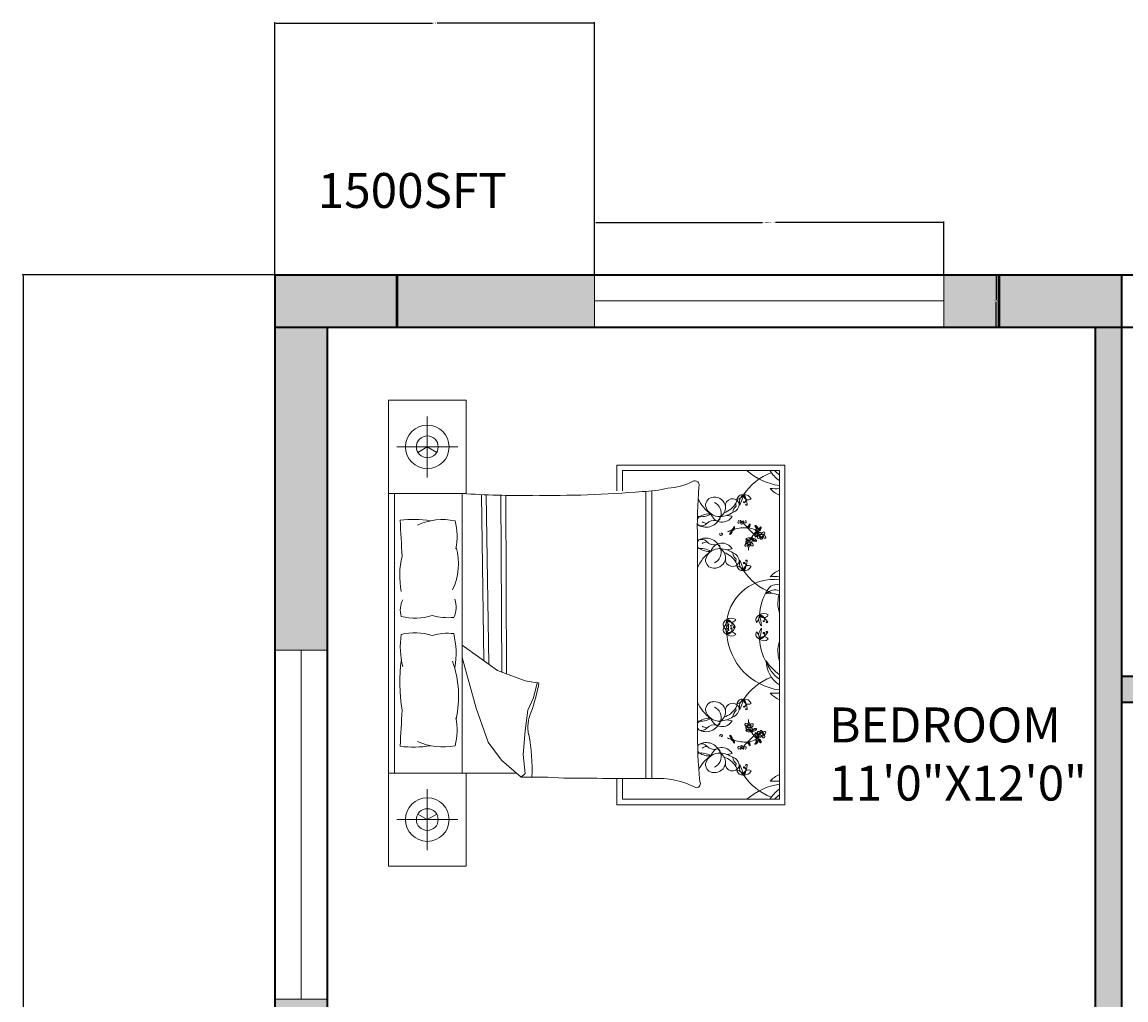
# Model space of a CAD drawing. Units: inches. Extents: x -28 to 485, y -861 to 54.
# Tile 10 of 14: x -28 to 162, y -115 to 54. Entities that reach past the tile are written whole.
import ezdxf

# ---------------------------------------------------------------- set-up
doc = ezdxf.new("R2010")
doc.units = ezdxf.units.IN
doc.header["$MEASUREMENT"] = 0
for name, color, linetype, lineweight in [('A-ANNO-DIMS', 2, 'Continuous', 18), ('A-AREA-IDEN', 7, 'Continuous', 18), ('A-COLS', 7, 'Continuous', 50), ('A-COLS-PATT', 8, 'Continuous', 13), ('A-FURN', 8, 'Continuous', 13), ('A-GLAZ', 4, 'Continuous', 18), ('A-WALL', 7, 'Continuous', 35), ('A-WALL-PATT', 34, 'Continuous', 13)]:
    doc.layers.add(name, color=color, linetype=linetype, lineweight=lineweight)
doc.styles.get("Standard").update_dxf_attribs({"font": 'arial.ttf'})
doc.dimstyles.get("Standard").update_dxf_attribs({"dimtxt": 0.18, "dimasz": 0.18, "dimexe": 0.18, "dimexo": 0.0625, "dimgap": 0.09, "dimtad": 0, "dimtih": 1, "dimtoh": 1, "dimdec": 0, "dimzin": 0, "dimdsep": 46, "dimlunit": 3, "dimtxsty": 'Standard', "dimcen": 0.09, "dimadec": 0, "dimazin": 0, "dimtfac": 1, "dimtdec": 0, "dimtofl": 0, "dimtmove": 0, "dimatfit": 3, "dimfxl": 1, "dimtolj": 1, "dimtzin": 0, "dimarcsym": 0})

# ---------------------------------------------------------------- blocks, each defined once
blk = doc.blocks.new('BED-DOUBLE-WITH-NIGHTSTANDS')
for p, q in [((0, 0), (0, 80.08)), ((6.67, 66.84), (6.67, 77.31)), ((11.91, 72.08), (1.44, 72.08)), ((39.26, 64.51), (39.26, 68.96)), ((39.26, 68.96), (68.11, 68.96)), ((68.11, 68.96), (68.11, 10.57)), ((40.19, 68.03), (40.19, 64.5)), ((67.18, 68.03), (40.19, 68.03)), ((67.18, 11.5), (67.18, 68.03)), ((45.25, 64.51), (45.25, 15.09)), ((1.03, 64.07), (1.03, 16.02)), ((12.66, 16.02), (12.66, 64.07)), ((15.98, 63.85), (16.38, 35.34)), ((16.8, 63.82), (17.22, 34.74)), ((19.33, 63.78), (19.45, 33.37)), ((20.15, 63.78), (20.27, 33.06)), ((44.25, 64.43), (44.25, 15.09)), ((59.06, 60.14), (58.15, 60.31)), ((53.12, 56.3), (53.12, 23.78)), ((59.06, 54.54), (58.15, 54.36)), ((12.66, 38.02), (18.76, 33.63)), ((15.04, 27.14), (12.66, 35.87)), ((18.76, 33.63), (23.47, 31.84)), ((23.47, 31.84), (25.57, 31.52)), ((25.57, 31.52), (24.92, 28.93)), ((24.92, 28.93), (23.95, 26.82)), ((17.14, 21.3), (15.04, 27.14)), ((23.95, 26.82), (23.47, 23.25)), ((59.06, 24.99), (58.15, 25.16)), ((23.47, 23.25), (23.14, 19.19)), ((19.41, 18.22), (17.14, 21.3)), ((23.14, 19.19), (23.47, 15.95)), ((59.06, 19.39), (58.15, 19.21)), ((22.82, 15.3), (19.41, 18.22)), ((0, 16.02), (21.98, 16.02)), ((23.47, 15.95), (22.82, 15.3)), ((39.26, 10.57), (39.26, 15.1)), ((40.19, 15.1), (40.19, 11.5)), ((6.67, 13.24), (6.67, 2.78)), ((40.19, 11.5), (67.18, 11.5)), ((68.11, 10.57), (39.26, 10.57)), ((11.91, 8.01), (1.44, 8.01))]:
    blk.add_line(p, q)
for points in [[(0, 64.07), (13.35, 64.07), (13.35, 80.08), (0, 80.08)], [(6.67, 72.08), (5.06, 71.14)], [(6.67, 72.08), (8.29, 71.14)], [(13.35, 16.02), (13.35, 0), (0, 0)], [(6.67, 8.01), (5.06, 8.94)], [(6.67, 8.01), (8.29, 8.94)]]:
    blk.add_lwpolyline(points)
for points in [[(43.62, 64.41, 0.056112), (48.03, 64.99, 0.095341), (52.27, 66.12)], [(2, 59.47, -0.074897), (7.23, 59.37, 0.472817)], [(7.52, 43.09, -0.14099), (2.18, 42.93, -0.235245)], [(7.52, 39.67, 0.14099), (2.18, 39.83, 0.235245)], [(2, 20.62, 0.074897), (7.23, 20.71, -0.472817)], [(30.15, 15.13, 0.001242), (45.35, 15.09, -0.127202), (52.92, 13.49)]]:
    blk.add_lwpolyline(points, format="xyb")
for centre, radius in [((6.67, 72.08), 3.74), ((6.67, 72.08), 1.87), ((64.11, 56.84), 0.204), ((61.96, 55.51), 0.204), ((61.96, 24.02), 0.204), ((64.11, 22.68), 0.204), ((6.67, 8.01), 3.74), ((6.67, 8.01), 1.87)]:
    blk.add_circle(centre, radius)
for centre, radius, start, end in [((69.62, 57.92), 10.46, 111.4092, 145.6135), ((68.59, 75.81), 10.46, 228.1144, 262.255), ((69.99, 70.57), 5.1, 209.8884, 236.5383), ((70.94, 72.4), 6.35, 223.5186, 233.6964), ((52.68, 65.51), 0.73, 336.5219, 123.8264), ((131.01, 58.75), 77.93, 175.2402, 181.8035), ((68.81, 67.71), 4.25, 221.0454, 247.4453), ((66.52, 79.36), 14.47, 266.3481, 272.5919), ((22.44, 207.63), 143.9, 266.1, 270.9282), ((27.68, 251.44), 187.71, 269.1145, 274.8735), ((58.76, 65.61), 6.06, 203.6453, 236.3329), ((55.85, 62.08), 1.35, 88.9462, 185.5144), ((56.04, 61.53), 1.91, 7.1143, 95.0551), ((59.12, 61.97), 1.2, 19.1312, 189.736), ((60.43, 62.21), 0.737, 126.7319, 206.0245), ((60.79, 62.99), 0.867, 76.272, 177.0484), ((59.47, 64.76), 1.79, 284.7031, 328.6173), ((61.96, 62.49), 1.65, 125.7657, 194.5347), ((53.85, 65.41), 7.32, 332.8176, 347.4827), ((61.24, 62.69), 1.16, 20.9613, 102.2885), ((61.86, 63.85), 0.873, 181.7131, 301.5367), ((59, 62.09), 2.64, 2.0648, 41.1598), ((60.59, 63.07), 0.856, 316.2238, 62.3173), ((61.09, 62.57), 0.0682, 20.2667, 316.2271), ((56.85, 62.5), 2.41, 193.079, 274.7067), ((55.32, 60.77), 1.86, 338.5779, 68.4181), ((55.62, 61.86), 2.33, 305.9599, 357.6409), ((56.78, 64.39), 4.3, 273.4924, 303.7117), ((56.48, 64.35), 3.78, 288.2955, 328.7386), ((58.76, 62.26), 1.5, 285.6955, 4.031), ((60.76, 60.64), 1.6, 128.4175, 173.8338), ((61.51, 62.18), 0.13, 168.5166, 2.0648), ((61.45, 62.19), 0.0631, 52.0591, 168.5166), ((-760.15, 15.33), 763.42, 2.85022, 3.31479), ((9.33, 49.26), 10.32, 78.2417, 114.8684), ((1.06, 56.61), 10.73, 348.9631, 14.8961), ((54, 59.28), 0.964, 127.675, 162.5814), ((54, 59.28), 0.964, 196.6343, 225.5483), ((53.71, 63.39), 3.32, 259.249, 301.1782), ((54.57, 60.82), 2.55, 240.8249, 340.7178), ((53.81, 59.69), 1.2, 246.1646, 318.4347), ((55.15, 57.49), 3.09, 85.2696, 124.215), ((55.03, 61.2), 2.3, 240.0851, 262.564), ((55.94, 57.8), 1.64, 74.8529, 138.4347), ((57.33, 61.13), 1.99, 196.8663, 330.0915), ((56.5, 59.87), 0.497, 254.8529, 12.6959), ((55.15, 57.49), 3.09, 53.6555, 57.2989), ((60.19, 59.12), 0.158, 125.0752, 284.7644), ((60.43, 59.18), 0.34, 127.3642, 168.4363), ((60.17, 59.45), 0.49, 277.4968, 341.2737), ((60.56, 59.22), 0.195, 88.1325, 178.8919), ((60.95, 59.02), 0.422, 136.3462, 189.6513), ((60.71, 58.98), 0.176, 189.6513, 312.3208), ((60.75, 59.46), 0.204, 183.2768, 356.7232), ((61.39, 59.1), 0.668, 164.2829, 186.9148), ((60.6, 59.09), 0.334, 312.3208, 40.2111), ((61.31, 59.47), 0.474, 201.6382, 274.947), ((60.68, 58.82), 0.619, 42.3896, 66.5724), ((66.93, 63.72), 7.6, 217.9541, 226.8459), ((61.13, 59.18), 0.337, 10.9597, 52.2379), ((61.33, 59.15), 0.156, 274.947, 37.5263), ((62.33, 58.47), 0.42, 115.5379, 168.6744), ((60.9, 59.07), 1.27, 329.344, 349.7412), ((59.89, 58.78), 2.26, 352.8698, 1.6736), ((57.16, 57.12), 0.251, 169.5864, 349.5616), ((57.25, 57.11), 0.154, 349.5616, 167.2949), ((61.28, 51.56), 6.63, 110.1059, 116.9968), ((59.06, 57.02), 0.42, 129.5056, 182.6421), ((57.85, 58), 1.27, 308.4388, 328.836), ((57.63, 59.02), 2.26, 296.5064, 305.3102), ((57.61, 57.86), 1.29, 336.3901, 344.4871), ((59.01, 57.53), 0.163, 83.9457, 185.6216), ((58.36, 57.69), 0.671, 328.836, 0.8141), ((58.71, 57.49), 0.384, 306.5232, 32.4668), ((59.16, 57.79), 0.163, 112.5583, 214.2343), ((59.06, 58.08), 0.384, 265.7131, 351.6568), ((58.72, 58.29), 0.671, 297.3659, 329.344), ((58.21, 58.87), 1.29, 313.6929, 321.7899), ((59.64, 57.99), 0.42, 115.5379, 168.6744), ((58.21, 58.6), 1.27, 329.344, 349.7412), ((61.28, 51.56), 6.63, 86.1723, 106.4158), ((57.2, 58.31), 2.26, 352.8698, 1.6736), ((61.86, 58.27), 0.163, 112.5583, 214.2343), ((61.75, 58.56), 0.384, 265.7131, 351.6568), ((61.42, 58.77), 0.671, 297.3659, 329.344), ((61.45, 54.86), 3.33, 60.7959, 85.244), ((54.37, 50.07), 10.94, 37.8256, 47.7588), ((60.91, 59.35), 1.29, 313.6929, 321.7899), ((65.87, 54.52), 3.99, 130.182, 149.456), ((63.07, 58.33), 0.228, 33.0979, 123.1364), ((58.05, 55.12), 5.96, 31.1156, 34.8118), ((62.74, 57.94), 0.617, 2.3172, 70.5201), ((63.67, 56.79), 0.658, 139.3812, 199.9959), ((62.44, 57.27), 0.93, 310.9365, 22.7695), ((63.25, 57.78), 0.178, 135.7354, 318.1297), ((62.95, 58.07), 0.236, 315.7354, 31.1156), ((62.75, 57.57), 0.547, 319.3812, 5.5456), ((63.38, 57.79), 0.178, 68.2452, 250.6395), ((62.97, 58), 0.531, 352.6008, 57.1845), ((64.87, 54.44), 3.55, 111.7087, 116.2181), ((61.45, 54.86), 3.33, 47.5083, 55.9967), ((63.48, 58.12), 0.531, 252.8042, 349.6943), ((62.97, 57.17), 0.565, 331.1838, 51.6792), ((63.53, 58.17), 0.236, 248.2452, 323.6254), ((63.33, 58.31), 0.617, 291.7087, 3.0299), ((63.75, 57.1), 0.2, 138.2946, 276.2474), ((63.83, 57.07), 0.278, 358.5719, 143.8954), ((58.93, 61.56), 5.96, 323.6254, 327.3216), ((63.99, 57.29), 0.281, 208.8493, 269.9355), ((63.75, 57.22), 0.321, 274.2123, 318.1587), ((63.81, 58.16), 0.228, 325.6077, 55.6462), ((64.73, 56.9), 0.643, 121.9501, 165.2442), ((64.28, 57.14), 0.135, 262.868, 7.094), ((64.27, 57.26), 0.403, 278.5614, 22.5914), ((64.49, 57.27), 0.202, 44.3732, 121.9501), ((54, 55.39), 0.964, 134.4517, 156.7144), ((54.57, 53.85), 2.55, 19.2822, 119.1751), ((53.81, 54.99), 1.2, 41.5653, 113.8354), ((55.03, 53.47), 2.3, 97.436, 119.9149), ((55.94, 56.87), 1.64, 221.5653, 285.1471), ((57.33, 53.55), 1.99, 29.9085, 163.1337), ((56.5, 54.81), 0.497, 347.3041, 105.1471), ((61.4, 55.17), 0.158, 125.0752, 284.7644), ((61.65, 55.23), 0.34, 93.635, 168.4363), ((61.66, 57.07), 0.93, 253.6301, 325.4631), ((61.92, 55.78), 0.658, 82.0748, 142.6895), ((61.85, 56.68), 0.675, 228.342, 274.9894), ((61.6, 55.76), 0.2, 138.2946, 276.2474), ((61.38, 55.5), 0.49, 277.4968, 341.2737), ((61.68, 55.73), 0.278, 358.5719, 143.8954), ((61.77, 55.27), 0.195, 88.1325, 178.8919), ((61.84, 55.95), 0.281, 208.8493, 269.9355), ((61.6, 55.89), 0.321, 274.2123, 318.1587), ((62.16, 55.06), 0.422, 136.3462, 189.6513), ((61.87, 56.57), 0.565, 273.8774, 357.1501), ((62.6, 55.14), 0.668, 164.2829, 186.9148), ((62.58, 55.56), 0.643, 121.9501, 165.2442), ((62.09, 56.97), 0.547, 262.0748, 308.2393), ((61.81, 55.14), 0.334, 312.3208, 40.2111), ((62.52, 55.52), 0.474, 201.6382, 274.947), ((62.13, 55.81), 0.135, 262.868, 7.094), ((61.89, 54.87), 0.619, 42.3896, 66.5724), ((62.12, 55.92), 0.403, 278.5614, 22.5914), ((62.34, 55.23), 0.337, 10.9597, 118.7804), ((65.87, 54.52), 3.99, 156.1523, 156.9499), ((62.34, 55.94), 0.202, 44.3732, 121.9501), ((62.97, 56.41), 0.565, 181.4625, 249.4747), ((62.87, 56.86), 0.547, 215.1128, 261.2773), ((63.31, 56.83), 0.93, 197.889, 269.722), ((62.55, 55.2), 0.156, 274.947, 37.5263), ((63.02, 56.51), 0.675, 248.3627, 295.0101), ((62.69, 55.67), 0.658, 20.6625, 81.2773), ((62.87, 57.22), 0.675, 285.6484, 332.2957), ((63.55, 56.5), 0.158, 125.0752, 284.7644), ((63.8, 56.56), 0.34, 93.635, 168.4363), ((63.53, 56.83), 0.49, 277.4968, 341.2737), ((63.92, 56.61), 0.195, 88.1325, 178.8919), ((64.31, 56.4), 0.422, 136.3462, 189.6513), ((64.07, 56.36), 0.176, 189.6513, 312.3208), ((64.75, 56.48), 0.668, 164.2829, 186.9148), ((63.96, 56.47), 0.334, 312.3208, 40.2111), ((64.67, 56.85), 0.474, 201.6382, 274.947), ((64.04, 56.2), 0.619, 42.3896, 66.5724), ((64.49, 56.56), 0.337, 10.9597, 118.7804), ((64.7, 56.53), 0.156, 274.947, 37.5263), ((16.01, 49.96), 14.08, 166.3427, 191.1841), ((1.85, 51.98), 10.19, 333.8761, 16.1746), ((54, 55.39), 0.964, 203.2856, 232.325), ((53.71, 51.28), 3.32, 58.8218, 100.2867), ((58.76, 49.06), 6.06, 123.6671, 158.5059), ((55.15, 57.18), 3.09, 235.785, 274.7304), ((56.85, 52.18), 2.41, 85.2933, 166.921), ((55.32, 53.9), 1.86, 291.5819, 21.4221), ((55.15, 57.18), 3.09, 302.7011, 306.3445), ((55.62, 52.81), 2.33, 2.3591, 54.0401), ((56.78, 50.29), 4.3, 56.2883, 86.5076), ((56.48, 50.32), 3.78, 31.2614, 71.7045), ((60.76, 54.03), 1.6, 186.1662, 231.5825), ((58.76, 52.42), 1.5, 355.969, 74.3045), ((61.92, 55.02), 0.176, 189.6513, 312.3208), ((65.87, 54.52), 3.99, 175.2415, 182.8929), ((55.85, 52.59), 1.35, 174.4856, 271.0538), ((56.04, 53.15), 1.91, 264.9449, 352.8857), ((59.12, 52.71), 1.2, 170.264, 340.8688), ((60.43, 52.46), 0.737, 153.9755, 233.2681), ((60.79, 51.69), 0.867, 182.9516, 283.728), ((59.47, 49.92), 1.79, 31.3827, 75.2969), ((61.96, 52.19), 1.65, 165.4653, 234.2343), ((53.85, 49.26), 7.32, 12.5173, 27.1824), ((59, 52.59), 2.64, 318.8402, 357.9352), ((60.59, 51.6), 0.856, 297.6827, 43.7762), ((61.86, 50.82), 0.873, 58.4633, 178.2869), ((61.24, 51.98), 1.16, 257.7115, 339.0387), ((61.13, 52.12), 0.113, 43.7762, 339.7183), ((61.51, 52.5), 0.13, 357.9352, 191.4834), ((61.45, 52.48), 0.0631, 191.4834, 307.9409), ((69.62, 56.75), 10.46, 214.3865, 248.5908), ((68.81, 46.96), 4.25, 112.5547, 138.9546), ((66.52, 35.31), 14.47, 87.4081, 93.6519), ((66.17, 41.19), 8.09, 82.8636, 171.8197), ((66.74, 46.53), 1.88, 76.3898, 169.0739), ((66.48, 45.12), 2.37, 72.8609, 131.9049), ((5.99, 44.03), 3.96, 153.3437, 196.1026), ((7.37, 44.56), 4.25, 335.0183, 18.5407), ((74.19, 42.33), 10.46, 152.5854, 175.5377), ((65.43, 42.24), 4.68, 68.117, 96.6195), ((72.68, 45.26), 5.75, 162.9798, 196.4569), ((75.64, 42.98), 8.5, 174.3643, 175.6213), ((81.47, 38.5), 15.2, 160.0972, 160.2783), ((10.2, 52.53), 9.81, 254.1707, 275.9871), ((58.4, 41.51), 0.867, 106.1963, 206.9726), ((56.38, 42.39), 1.79, 314.6273, 358.5415), ((59.67, 41.66), 1.65, 155.6899, 224.4589), ((58.94, 41.49), 1.16, 50.8855, 132.2127), ((58.91, 42.8), 0.873, 211.6373, 331.4609), ((58.2, 41.49), 0.856, 346.148, 92.2415), ((57.3, 39.84), 2.64, 31.989, 71.0841), ((51.18, 40.16), 7.32, 2.7418, 17.407), ((64.01, 42.31), 0.867, 106.1963, 206.9726), ((61.98, 43.19), 1.79, 314.6273, 358.5415), ((65.27, 42.46), 1.65, 155.6899, 224.4589), ((64.54, 42.29), 1.16, 50.8855, 132.2127), ((64.51, 43.6), 0.873, 211.6373, 331.4609), ((63.8, 42.29), 0.856, 346.148, 92.2415), ((62.91, 40.64), 2.64, 31.989, 71.0841), ((56.78, 40.96), 7.32, 2.7418, 17.407), ((64.47, 42.1), 0.0682, 50.1909, 346.0209), ((64.98, 41.95), 0.0631, 81.9833, 198.4408), ((65.04, 41.98), 0.13, 198.4408, 31.989), ((10.2, 30.23), 9.81, 84.0129, 105.8293), ((-2.51, 36.66), 14.12, 349.8617, 13.6238), ((58.4, 40.68), 0.867, 153.0274, 253.8037), ((56.38, 39.81), 1.79, 1.4585, 45.3727), ((59.67, 40.53), 1.65, 135.5411, 204.3101), ((51.18, 42.04), 7.32, 342.593, 357.2582), ((57.3, 42.35), 2.64, 288.9159, 328.011), ((58.2, 40.71), 0.856, 267.7585, 13.852), ((58.91, 39.39), 0.873, 28.5391, 148.3627), ((58.94, 40.71), 1.16, 227.7873, 309.1145), ((68.59, 40.66), 10.46, 184.4623, 262.255), ((58.87, 41.3), 0.0682, 50.1909, 346.0209), ((58.92, 40.88), 0.113, 13.852, 309.9245), ((59.44, 41.17), 0.13, 198.4408, 31.989), ((59.37, 41.15), 0.0631, 81.9833, 198.4408), ((59.44, 41.02), 0.13, 328.011, 161.5592), ((59.37, 41.04), 0.0631, 161.5592, 278.0167), ((64.01, 39.88), 0.867, 153.0274, 253.8037), ((61.98, 39.01), 1.79, 1.4585, 45.3727), ((65.27, 39.73), 1.65, 135.5411, 204.3101), ((56.78, 41.24), 7.32, 342.593, 357.2582), ((62.91, 41.55), 2.64, 288.9159, 328.011), ((63.8, 39.91), 0.856, 267.7585, 13.852), ((64.52, 40.08), 0.113, 13.852, 309.9245), ((64.98, 40.24), 0.0631, 161.5592, 278.0167), ((65.04, 40.22), 0.13, 328.011, 161.5592), ((16.3, 37.72), 14.27, 171.5249, 193.96), ((64.51, 38.59), 0.873, 28.5391, 148.3627), ((64.54, 39.91), 1.16, 227.7873, 309.1145), ((74.19, 39.86), 10.46, 184.4623, 207.4146), ((72.68, 36.94), 5.75, 163.5431, 197.0202), ((75.64, 39.22), 8.5, 184.3787, 185.6357), ((81.47, 43.7), 15.2, 199.7217, 199.9028), ((30.98, 31.59), 29.04, 172.2196, 189.497), ((-6.57, 29.12), 18.61, 348.0397, 19.2615), ((69.99, 35.42), 5.1, 181.272, 236.5383), ((72.72, 40.59), 9.45, 214.0123, 234.053), ((70.94, 37.25), 6.35, 197.8504, 233.6964), ((69.62, 22.77), 10.46, 111.4092, 145.6135), ((-4.69, 37.08), 31.06, 340.1194, 349.3383), ((25.64, 31.34), 0.193, 358.8623, 109.7536), ((60.79, 27.84), 0.867, 76.272, 177.0484), ((59.47, 29.61), 1.79, 284.7031, 328.6173), ((61.96, 27.34), 1.65, 125.7657, 194.5347), ((53.85, 30.27), 7.32, 332.8176, 347.4827), ((61.24, 27.55), 1.16, 20.9613, 102.2885), ((60.59, 27.92), 0.856, 316.2238, 62.3173), ((59, 26.94), 2.64, 2.0648, 41.1598), ((61.86, 28.71), 0.873, 181.7131, 301.5367), ((66.52, 44.21), 14.47, 266.3481, 272.5919), ((68.81, 32.56), 4.25, 221.0454, 247.4453), ((-760.15, 64.76), 763.42, 356.68521, 357.14978), ((58.76, 30.46), 6.06, 201.4941, 236.3329), ((55.85, 26.93), 1.35, 88.9462, 185.5144), ((56.85, 27.35), 2.41, 193.079, 274.7067), ((56.04, 26.38), 1.91, 7.1143, 95.0551), ((55.32, 25.63), 1.86, 338.5779, 68.4181), ((55.62, 26.71), 2.33, 305.9599, 357.6409), ((56.48, 29.2), 3.78, 288.2955, 328.7386), ((59.12, 26.82), 1.2, 19.1312, 189.736), ((58.76, 27.11), 1.5, 285.6955, 4.031), ((60.76, 25.49), 1.6, 128.4175, 173.8338), ((60.43, 27.07), 0.737, 126.7319, 206.0245), ((61.09, 27.42), 0.0682, 20.2667, 316.2271), ((61.51, 27.03), 0.13, 168.5166, 2.0648), ((61.45, 27.04), 0.0631, 52.0591, 168.5166), ((1.06, 23.47), 10.73, 345.1039, 11.0369), ((30.48, 23.89), 6.52, 156.2616, 191.3392), ((53.71, 28.24), 3.32, 259.7133, 301.1782), ((54, 24.13), 0.964, 127.675, 156.7144), ((54.57, 25.67), 2.55, 240.8249, 340.7178), ((55.15, 22.34), 3.09, 85.2696, 124.215), ((57.33, 25.98), 1.99, 196.8663, 330.0915), ((56.5, 24.72), 0.497, 254.8529, 12.6959), ((55.15, 22.34), 3.09, 53.6555, 57.2989), ((56.78, 29.24), 4.3, 273.4924, 303.7117), ((61.92, 24.5), 0.176, 47.6792, 170.3487), ((65.87, 25.01), 3.99, 177.1071, 184.7585), ((136.48, 22.83), 83.37, 179.3433, 185.6887), ((54, 24.13), 0.964, 203.229, 225.5483), ((53.81, 24.54), 1.2, 246.1646, 318.4347), ((55.03, 26.06), 2.3, 240.0851, 262.564), ((55.94, 22.65), 1.64, 74.8529, 138.4347), ((61.4, 24.36), 0.158, 75.2356, 234.9248), ((61.65, 24.3), 0.34, 191.5637, 266.365), ((61.6, 23.76), 0.2, 83.7526, 221.7054), ((61.85, 22.84), 0.675, 85.0106, 131.658), ((61.66, 22.46), 0.93, 34.5369, 106.3699), ((61.92, 23.75), 0.658, 217.3105, 277.9252), ((61.38, 24.03), 0.49, 18.7263, 82.5032), ((61.68, 23.79), 0.278, 216.1046, 1.4281), ((61.77, 24.25), 0.195, 181.1081, 271.8675), ((61.84, 23.57), 0.281, 90.0645, 151.1507), ((61.6, 23.64), 0.321, 41.8413, 85.7877), ((62.16, 24.46), 0.422, 170.3487, 223.6538), ((61.87, 22.95), 0.565, 2.8499, 86.1226), ((62.6, 24.38), 0.668, 173.0852, 195.7171), ((62.58, 23.96), 0.643, 194.7558, 238.0499), ((62.09, 22.55), 0.547, 51.7607, 97.9252), ((61.81, 24.39), 0.334, 319.7889, 47.6792), ((62.52, 24.01), 0.474, 85.053, 158.3618), ((62.13, 23.71), 0.135, 352.906, 97.132), ((61.89, 24.66), 0.619, 293.4276, 317.6104), ((62.34, 24.29), 0.337, 241.2196, 349.0403), ((62.12, 23.6), 0.403, 337.4086, 81.4386), ((65.87, 25.01), 3.99, 203.0501, 203.8477), ((62.34, 23.59), 0.202, 238.0499, 315.6268), ((62.97, 23.11), 0.565, 110.5253, 178.5375), ((63.31, 22.7), 0.93, 90.278, 162.111), ((62.87, 22.67), 0.547, 98.7227, 144.8872), ((65.87, 25.01), 3.99, 210.544, 229.818), ((62.55, 24.33), 0.156, 322.4737, 85.053), ((63.02, 23.01), 0.675, 64.9899, 111.6373), ((62.69, 23.86), 0.658, 278.7227, 339.3375), ((63.67, 22.74), 0.658, 160.0041, 220.6188), ((62.44, 22.26), 0.93, 337.2305, 49.0635), ((62.87, 22.31), 0.675, 27.7043, 74.3516), ((63.55, 23.03), 0.158, 75.2356, 234.9248), ((63.8, 22.96), 0.34, 191.5637, 266.365), ((63.53, 22.69), 0.49, 18.7263, 82.5032), ((63.92, 22.92), 0.195, 181.1081, 271.8675), ((64.07, 23.17), 0.176, 47.6792, 170.3487), ((64.31, 23.13), 0.422, 170.3487, 223.6538), ((64.75, 23.05), 0.668, 173.0852, 195.7171), ((63.96, 23.05), 0.334, 319.7889, 47.6792), ((64.67, 22.68), 0.474, 85.053, 158.3618), ((64.04, 23.32), 0.619, 293.4276, 317.6104), ((64.49, 22.96), 0.337, 241.2196, 349.0403), ((64.7, 22.99), 0.156, 322.4737, 85.053), ((9.33, 30.82), 10.32, 245.1316, 281.7583), ((-5.54, 16.67), 30.23, 357.4519, 11.3392), ((54, 20.25), 0.964, 134.4517, 153.558), ((54.57, 18.71), 2.55, 19.2822, 119.1751), ((53.81, 19.84), 1.2, 41.5653, 113.8354), ((57.16, 22.4), 0.251, 10.4384, 190.4136), ((57.25, 22.42), 0.154, 192.7051, 10.4384), ((61.28, 27.97), 6.63, 243.0032, 249.8941), ((57.85, 21.53), 1.27, 31.164, 51.5612), ((59.06, 22.5), 0.42, 177.3579, 230.4944), ((57.63, 20.5), 2.26, 54.6898, 63.4936), ((57.61, 21.66), 1.29, 15.5129, 23.6099), ((59.01, 21.99), 0.163, 174.3784, 276.0543), ((58.71, 22.03), 0.384, 327.5332, 53.4768), ((58.36, 21.84), 0.671, 359.1859, 31.164), ((59.16, 21.74), 0.163, 145.7657, 247.4417), ((59.06, 21.45), 0.384, 8.3432, 94.2869), ((58.72, 21.23), 0.671, 30.656, 62.6341), ((58.21, 20.66), 1.29, 38.2101, 46.3071), ((59.64, 21.53), 0.42, 191.3256, 244.4621), ((58.21, 20.93), 1.27, 10.2588, 30.656), ((61.28, 27.97), 6.63, 253.5842, 273.8277), ((57.2, 21.22), 2.26, 358.3264, 7.1302), ((66.93, 15.8), 7.6, 133.1541, 142.0459), ((61.86, 21.26), 0.163, 145.7657, 247.4417), ((54.37, 29.45), 10.94, 312.2412, 322.1744), ((61.45, 24.67), 3.33, 274.756, 299.2041), ((61.75, 20.97), 0.384, 8.3432, 94.2869), ((61.42, 20.76), 0.671, 30.656, 62.6341), ((60.91, 20.18), 1.29, 38.2101, 46.3071), ((62.33, 21.06), 0.42, 191.3256, 244.4621), ((60.9, 20.45), 1.27, 10.2588, 30.656), ((59.89, 20.74), 2.26, 358.3264, 7.1302), ((62.74, 21.59), 0.617, 289.4799, 357.6828), ((58.05, 24.41), 5.96, 325.1882, 328.8844), ((63.07, 21.2), 0.228, 236.8636, 326.9021), ((63.25, 21.74), 0.178, 41.8703, 224.2646), ((62.95, 21.45), 0.236, 328.8844, 44.2646), ((62.75, 21.95), 0.547, 354.4544, 40.6188), ((63.38, 21.74), 0.178, 109.3605, 291.7548), ((62.97, 21.52), 0.531, 302.8155, 7.3992), ((64.87, 25.09), 3.55, 243.7819, 248.2913), ((61.45, 24.67), 3.33, 304.0033, 312.4917), ((62.97, 22.35), 0.565, 308.3208, 28.8162), ((63.48, 21.4), 0.531, 10.3057, 107.1958), ((63.53, 21.36), 0.236, 36.3746, 111.7548), ((63.75, 22.43), 0.2, 83.7526, 221.7054), ((63.33, 21.21), 0.617, 356.9701, 68.2913), ((63.83, 22.46), 0.278, 216.1046, 1.4281), ((58.93, 17.96), 5.96, 32.6784, 36.3746), ((63.99, 22.24), 0.281, 90.0645, 151.1507), ((63.75, 22.31), 0.321, 41.8413, 85.7877), ((63.81, 21.37), 0.228, 304.3538, 34.3923), ((64.73, 22.63), 0.643, 194.7558, 238.0499), ((64.28, 22.38), 0.135, 352.906, 97.132), ((64.27, 22.27), 0.403, 337.4086, 81.4386), ((64.49, 22.25), 0.202, 238.0499, 315.6268), ((54, 20.25), 0.964, 210.0293, 232.325), ((53.71, 16.14), 3.32, 58.8218, 99.1554), ((55.15, 22.04), 3.09, 235.785, 274.7304), ((55.03, 18.32), 2.3, 97.436, 119.9149), ((56.85, 17.03), 2.41, 85.2933, 166.921), ((55.94, 21.72), 1.64, 221.5653, 285.1471), ((57.33, 18.4), 1.99, 29.9085, 163.1337), ((55.32, 18.75), 1.86, 291.5819, 21.4221), ((56.5, 19.66), 0.497, 347.3041, 105.1471), ((55.15, 22.04), 3.09, 302.7011, 306.3445), ((55.62, 17.67), 2.33, 2.3591, 54.0401), ((56.78, 15.14), 4.3, 56.2883, 86.5076), ((60.19, 20.41), 0.158, 75.2356, 234.9248), ((60.43, 20.35), 0.34, 191.5637, 232.6358), ((60.17, 20.07), 0.49, 18.7263, 82.5032), ((60.56, 20.3), 0.195, 181.1081, 271.8675), ((60.71, 20.55), 0.176, 47.6792, 170.3487), ((60.95, 20.51), 0.422, 170.3487, 223.6538), ((60.75, 20.06), 0.204, 3.2768, 176.7232), ((61.39, 20.43), 0.668, 173.0852, 195.7171), ((60.6, 20.43), 0.334, 319.7889, 47.6792), ((61.31, 20.06), 0.474, 85.053, 158.3618), ((60.68, 20.7), 0.619, 293.4276, 317.6104), ((61.13, 20.34), 0.337, 307.7621, 349.0403), ((61.33, 20.37), 0.156, 322.4737, 85.053), ((58.76, 13.91), 6.06, 123.6671, 153.2997), ((55.85, 17.44), 1.35, 174.4856, 271.0538), ((56.04, 18), 1.91, 264.9449, 352.8857), ((56.48, 15.18), 3.78, 31.2614, 71.7045), ((59.12, 17.56), 1.2, 170.264, 340.8688), ((58.76, 17.27), 1.5, 355.969, 74.3045), ((60.76, 18.89), 1.6, 186.1662, 231.5825), ((60.43, 17.31), 0.737, 153.9755, 233.2681), ((61.96, 17.04), 1.65, 165.4653, 234.2343), ((53.85, 14.11), 7.32, 12.5173, 27.1824), ((59, 17.44), 2.64, 318.8402, 357.9352), ((61.13, 16.97), 0.113, 43.7762, 339.7183), ((61.51, 17.35), 0.13, 357.9352, 191.4834), ((61.45, 17.33), 0.0631, 191.4834, 307.9409), ((24.81, -58.13), 73.46, 85.8294, 91.553), ((59.47, 14.77), 1.79, 31.3827, 75.2969), ((60.79, 16.54), 0.867, 182.9516, 283.728), ((60.59, 16.46), 0.856, 297.6827, 43.7762), ((61.86, 15.67), 0.873, 58.4633, 178.2869), ((61.24, 16.83), 1.16, 257.7115, 339.0387), ((69.62, 21.6), 10.46, 214.3865, 248.5908), ((68.81, 11.81), 4.25, 112.5547, 138.9546), ((52.87, 14.23), 0.739, 273.98, 27.3412), ((68.59, 3.71), 10.46, 97.745, 131.8856), ((66.52, 0.17), 14.47, 87.4081, 93.6519), ((69.99, 8.96), 5.1, 123.4617, 150.1116), ((70.94, 7.13), 6.35, 126.3036, 136.4814)]:
    blk.add_arc(centre, radius, start, end)
blk = doc.blocks.new('WINDOW-60IN')
for p, q in [((0, 60), (0, 0)), ((9, 60), (0, 60)), ((4.5, 60), (4.5, 0)), ((9, 0), (9, 60)), ((0, 0), (9, 0))]:
    blk.add_line(p, q)
blk = doc.blocks.new('*D20')
at = {"layer": 'A-ANNO-DIMS', "color": 0, "lineweight": -2, "transparency": 16777216}
for p, q in [((70.24, 10.2), (70.24, 19.31)), ((70.42, 19.13), (99.12, 19.13)), ((130.06, 19.13), (101.35, 19.13)), ((130.24, 10.2), (130.24, 19.31))]:
    blk.add_line(p, q, dxfattribs=at)
at = {"layer": 'A-ANNO-DIMS', "color": 0, "transparency": 16777216}
for points in [[(70.42, 19.16), (70.42, 19.1), (70.24, 19.13)], [(130.06, 19.16), (130.06, 19.1), (130.24, 19.13)]]:
    blk.add_solid(points, dxfattribs=at)
at = {"layer": 'Defpoints', "color": 0, "transparency": 16777216}
for p in [(70.24, 19.13), (70.24, 10.13), (130.24, 10.13)]:
    blk.add_point(p, dxfattribs=at)
at = {"layer": 'A-ANNO-DIMS', "color": 0, "transparency": 16777216, "insert": (100.24, 19.13), "char_height": 0.18, "attachment_point": 5}
blk.add_mtext('\\A1;WINDOW 60 TYP.', dxfattribs=at)
blk = doc.blocks.new('*D21')
at = {"layer": 'A-ANNO-DIMS', "color": 0, "lineweight": -2, "transparency": 16777216}
for p, q in [((130.3, 10.13), (139.42, 10.13)), ((139.24, 9.95), (139.24, 5.82)), ((139.24, 1.31), (139.24, 5.45)), ((130.3, 1.13), (139.42, 1.13))]:
    blk.add_line(p, q, dxfattribs=at)
at = {"layer": 'A-ANNO-DIMS', "color": 0, "transparency": 16777216}
for points in [[(139.21, 9.95), (139.27, 9.95), (139.24, 10.13)], [(139.21, 1.31), (139.27, 1.31), (139.24, 1.13)]]:
    blk.add_solid(points, dxfattribs=at)
at = {"layer": 'Defpoints', "color": 0, "transparency": 16777216}
for p in [(130.24, 10.13), (139.24, 10.13), (130.24, 1.13)]:
    blk.add_point(p, dxfattribs=at)
at = {"layer": 'A-ANNO-DIMS', "color": 0, "transparency": 16777216, "insert": (139.24, 5.63), "char_height": 0.18, "attachment_point": 5}
blk.add_mtext('\\A1;9 TYP.', dxfattribs=at)
blk = doc.blocks.new('*D54')
at = {"layer": 'A-ANNO-DIMS', "color": 0, "lineweight": -2, "transparency": 16777216}
for p, q in [((15.22, 10.13), (-28.15, 10.13)), ((-27.97, 9.95), (-27.97, -177.18)), ((-27.97, -364.69), (-27.97, -177.55)), ((15.22, -364.87), (-28.15, -364.87))]:
    blk.add_line(p, q, dxfattribs=at)
at = {"layer": 'A-ANNO-DIMS', "color": 0, "transparency": 16777216}
for points in [[(-28, 9.95), (-27.94, 9.95), (-27.97, 10.13)], [(-28, -364.69), (-27.94, -364.69), (-27.97, -364.87)]]:
    blk.add_solid(points, dxfattribs=at)
at = {"layer": 'Defpoints', "color": 0, "transparency": 16777216}
for p in [(15.28, 10.13), (-27.97, -364.87), (15.28, -364.87)]:
    blk.add_point(p, dxfattribs=at)
at = {"layer": 'A-ANNO-DIMS', "color": 0, "transparency": 16777216, "insert": (-27.97, -177.37), "char_height": 0.18, "attachment_point": 5}
blk.add_mtext('\\A1;375', dxfattribs=at)
blk = doc.blocks.new('*D57')
at = {"layer": 'A-ANNO-DIMS', "color": 0, "lineweight": -2, "transparency": 16777216}
for p, q in [((15.28, 10.2), (15.28, 53.56)), ((15.46, 53.38), (42.37, 53.38)), ((70.06, 53.38), (43.15, 53.38)), ((70.24, 10.2), (70.24, 53.56))]:
    blk.add_line(p, q, dxfattribs=at)
at = {"layer": 'A-ANNO-DIMS', "color": 0, "transparency": 16777216}
for points in [[(15.46, 53.41), (15.46, 53.35), (15.28, 53.38)], [(70.06, 53.41), (70.06, 53.35), (70.24, 53.38)]]:
    blk.add_solid(points, dxfattribs=at)
at = {"layer": 'Defpoints', "color": 0, "transparency": 16777216}
for p in [(70.24, 53.38), (15.28, 10.13), (70.24, 10.13)]:
    blk.add_point(p, dxfattribs=at)
at = {"layer": 'A-ANNO-DIMS', "color": 0, "transparency": 16777216, "insert": (42.76, 53.38), "char_height": 0.18, "attachment_point": 5}
blk.add_mtext('\\A1;54.95', dxfattribs=at)

msp = doc.modelspace()

# ---------------------------------------------------------------- hatches: boundary and pattern name
at = {"layer": 'A-COLS-PATT'}
h = msp.add_hatch(color=256, dxfattribs=at)
h.dxf.hatch_style = 1
h.paths.add_polyline_path([(36.285, 10.133), (15.285, 10.133), (15.285, 1.133), (36.285, 1.133)])
h.paths.add_polyline_path([(160.785, 10.133), (139.785, 10.133), (139.785, 1.133), (160.785, 1.133)])
h.paths.add_polyline_path([(316.785, 10.133), (295.785, 10.133), (295.785, 1.133), (316.785, 1.133)])
h.paths.add_polyline_path([(441.285, 10.133), (420.285, 10.133), (420.285, 1.133), (441.285, 1.133)])
h.paths.add_polyline_path([(441.285, -138.367), (432.285, -138.367), (420.285, -138.367), (420.285, -147.367), (441.285, -147.367)])
h.paths.add_polyline_path([(304.785, -130.867), (295.785, -130.867), (295.785, -147.367), (304.785, -147.367), (304.785, -142.867)])
h.paths.add_polyline_path([(160.785, -130.867), (151.785, -130.867), (151.785, -142.867), (151.785, -147.367), (160.785, -147.367)])
h.paths.add_polyline_path([(36.285, -138.367), (24.285, -138.367), (15.285, -138.367), (15.285, -147.367), (36.285, -147.367)])
h.paths.add_polyline_path([(36.285, -355.867), (15.285, -355.867), (15.285, -364.867), (36.285, -364.867)])
h.paths.add_polyline_path([(160.785, -355.867), (139.785, -355.867), (139.785, -364.867), (160.785, -364.867)])
h.paths.add_polyline_path([(316.785, -355.867), (300.285, -355.867), (295.785, -355.867), (295.785, -364.867), (316.785, -364.867)])
at = {"layer": 'A-WALL-PATT'}
h = msp.add_hatch(color=256, dxfattribs=at)
h.dxf.hatch_style = 1
h.paths.add_polyline_path([(160.785, -808.867), (160.785, -817.867), (295.785, -817.867), (295.785, -808.867)])
h.paths.add_polyline_path([(316.785, -817.867), (323.776, -817.867), (323.776, -808.867), (316.785, -808.867)])
h.paths.add_polyline_path([(420.285, -817.867), (420.285, -808.867), (383.776, -808.867), (383.776, -817.867)])
h.paths.add_polyline_path([(432.285, -808.867), (441.285, -808.867), (441.285, -702.966), (432.285, -702.966), (432.285, -708.367), (397.785, -708.367), (397.785, -710.617), (397.785, -712.867), (432.285, -712.867)])
h.paths.add_polyline_path([(300.285, -712.867), (329.285, -712.867), (329.285, -710.617), (329.285, -708.367), (295.785, -708.367), (295.785, -808.867), (300.285, -808.867)])
h.paths.add_polyline_path([(160.785, -698.867), (158.535, -698.867), (156.285, -698.867), (156.285, -808.867), (160.785, -808.867)])
h.paths.add_polyline_path([(36.285, -808.867), (36.285, -817.867), (79.721, -817.867), (79.721, -808.867)])
h.paths.add_polyline_path([(15.285, -808.867), (24.285, -808.867), (24.285, -739.09), (15.285, -739.09)])
h.paths.add_polyline_path([(24.285, -640.781), (15.285, -640.781), (15.285, -679.09), (24.285, -679.09), (24.285, -664.867), (89.285, -664.867), (89.285, -662.617), (89.285, -660.367), (24.285, -660.367)])
h.paths.add_polyline_path([(15.285, -616.781), (24.285, -616.781), (24.285, -600.367), (15.285, -600.367)])
h.paths.add_polyline_path([(36.285, -595.867), (36.285, -600.367), (123.285, -600.367), (123.285, -660.367), (117.285, -660.367), (117.285, -664.867), (156.285, -664.867), (156.285, -670.867), (160.785, -670.867), (160.785, -660.367), (127.785, -660.367), (127.785, -600.367), (129.785, -600.367), (129.785, -598.117), (129.785, -595.867)])
h.paths.add_polyline_path([(367.785, -664.867), (363.285, -664.867), (363.285, -708.367), (357.285, -708.367), (357.285, -712.867), (369.785, -712.867), (369.785, -708.367), (367.785, -708.367)])
h.paths.add_polyline_path([(432.285, -664.867), (432.285, -666.966), (441.285, -666.966), (441.285, -642.367), (432.285, -642.367), (432.285, -660.367), (328.785, -660.367), (328.785, -664.867), (363.285, -664.867)])
h.paths.add_polyline_path([(333.285, -600.367), (420.285, -600.367), (420.285, -595.867), (326.785, -595.867), (326.785, -600.367), (328.785, -600.367), (328.785, -630.367), (331.035, -630.367), (333.285, -630.367)])
h.paths.add_polyline_path([(441.285, -600.367), (432.285, -600.367), (432.285, -618.367), (441.285, -618.367)])
h.paths.add_polyline_path([(432.285, -591.367), (441.285, -591.367), (441.285, -547.793), (432.285, -547.793)])
h.paths.add_polyline_path([(295.785, -588.367), (300.238, -588.367), (300.285, -583.867), (300.285, -451.867), (295.785, -451.867)])
h.paths.add_polyline_path([(420.285, -451.867), (420.285, -442.867), (316.785, -442.867), (316.785, -451.867)])
h.paths.add_polyline_path([(432.285, -487.793), (441.285, -487.793), (441.285, -451.867), (432.285, -451.867)])
h.paths.add_polyline_path([(432.285, -442.867), (441.285, -442.867), (441.285, -364.867), (432.285, -364.867)])
h.paths.add_polyline_path([(261.785, -451.867), (261.785, -447.367), (261.785, -444.758), (261.785, -442.867), (160.785, -442.867), (160.785, -451.867)])
h.paths.add_polyline_path([(139.785, -451.867), (139.785, -442.867), (36.285, -442.867), (36.285, -451.867)])
h.paths.add_polyline_path([(15.285, -491.617), (24.285, -491.617), (24.285, -451.867), (15.285, -451.867)])
h.paths.add_polyline_path([(24.285, -551.617), (15.285, -551.617), (15.285, -591.367), (24.285, -591.367)])
h.paths.add_polyline_path([(160.785, -451.867), (156.285, -451.867), (156.285, -588.367), (160.785, -588.367)])
h.paths.add_polyline_path([(139.785, -364.867), (139.785, -355.867), (36.285, -355.867), (36.285, -364.867)])
h.paths.add_polyline_path([(24.285, -364.867), (15.285, -364.867), (15.285, -373.867), (24.285, -373.867)])
h.paths.add_polyline_path([(15.285, -433.867), (15.285, -442.867), (24.285, -442.867), (24.285, -433.867)])
h.paths.add_polyline_path([(261.785, -364.867), (261.785, -360.367), (261.785, -355.867), (160.785, -355.867), (160.785, -364.867)])
h.paths.add_polyline_path([(295.785, -355.867), (289.785, -355.867), (289.785, -364.867), (295.785, -364.867)])
h.paths.add_polyline_path([(295.785, -355.867), (300.285, -355.867), (300.285, -259.867), (333.285, -259.867), (333.285, -257.617), (333.285, -255.367), (300.285, -255.367), (300.285, -207.367), (295.785, -207.367)])
h.paths.add_polyline_path([(420.285, -364.867), (420.285, -355.867), (316.785, -355.867), (316.785, -364.867)])
h.paths.add_polyline_path([(24.285, -311.192), (15.285, -311.192), (15.285, -355.867), (24.285, -355.867)])
h.paths.add_polyline_path([(24.285, -211.867), (54.144, -211.867), (54.144, -207.367), (24.285, -207.367), (24.285, -187.772), (15.285, -187.772), (15.285, -251.192), (24.285, -251.192)])
h.paths.add_polyline_path([(82.144, -207.367), (82.144, -209.617), (82.144, -211.867), (127.785, -211.867), (127.785, -147.367), (129.785, -147.367), (129.785, -145.117), (129.785, -142.867), (36.285, -142.867), (36.285, -147.367), (123.285, -147.367), (123.285, -207.367)])
h.paths.add_polyline_path([(160.785, -207.367), (156.285, -207.367), (156.285, -355.867), (160.785, -355.867)])
h.paths.add_polyline_path([(24.285, 1.133), (15.285, 1.133), (15.285, -54.408), (24.285, -54.408)])
h.paths.add_polyline_path([(36.285, 10.133), (36.285, 1.133), (70.235, 1.133), (70.235, 10.133)])
h.paths.add_polyline_path([(15.285, -138.367), (24.285, -138.367), (24.285, -114.408), (15.285, -114.408)])
h.paths.add_polyline_path([(24.285, -147.367), (15.285, -147.367), (15.285, -163.772), (24.285, -163.772)])
h.paths.add_polyline_path([(156.285, -130.867), (160.785, -130.867), (160.785, 1.133), (156.285, 1.133)])
h.paths.add_polyline_path([(130.235, 1.133), (139.785, 1.133), (139.785, 10.133), (130.235, 10.133)])
h.paths.add_polyline_path([(316.785, 10.133), (316.785, 1.133), (328.097, 1.133), (328.097, 10.133)])
h.paths.add_polyline_path([(300.285, 1.133), (295.785, 1.133), (295.785, -130.867), (300.285, -130.867)])
h.paths.add_polyline_path([(420.285, -147.367), (420.285, -142.867), (326.785, -142.867), (326.785, -145.117), (326.785, -147.367), (328.785, -147.367), (328.785, -177.367), (331.035, -177.367), (333.285, -177.367), (333.285, -147.367)])
h.paths.add_polyline_path([(333.285, -207.367), (333.285, -205.367), (328.785, -205.367), (328.785, -211.867), (363.285, -211.867), (363.285, -255.367), (361.285, -255.367), (361.285, -259.867), (369.785, -259.867), (369.785, -255.367), (367.785, -255.367), (367.785, -211.867), (432.285, -211.867), (432.285, -214.893), (441.285, -214.893), (441.285, -188.008), (432.285, -188.008), (432.285, -207.367)])
h.paths.add_polyline_path([(441.285, -250.893), (432.285, -250.893), (432.285, -255.367), (397.785, -255.367), (397.785, -257.617), (397.785, -259.867), (432.285, -259.867), (432.285, -355.867), (441.285, -355.867)])
h.paths.add_polyline_path([(432.285, -138.367), (441.285, -138.367), (441.285, -115.099), (432.285, -115.099)])
h.paths.add_polyline_path([(441.285, -147.367), (432.285, -147.367), (432.285, -164.008), (441.285, -164.008)])
h.paths.add_polyline_path([(420.285, 1.133), (420.285, 10.133), (388.097, 10.133), (388.097, 1.133)])
h.paths.add_polyline_path([(432.285, -55.099), (441.285, -55.099), (441.285, 1.133), (432.285, 1.133)])
h = msp.add_hatch(color=256, dxfattribs=at)
h.dxf.hatch_style = 1
h.paths.add_polyline_path([(196.785, -58.867), (160.785, -58.867), (160.785, -63.367), (196.785, -63.367)])
h.paths.add_polyline_path([(295.785, -58.867), (259.785, -58.867), (259.785, -63.367), (295.785, -63.367)])
h.paths.add_polyline_path([(196.785, -753.367), (160.785, -753.367), (160.785, -757.867), (196.785, -757.867)])
h.paths.add_polyline_path([(295.785, -753.367), (259.785, -753.367), (259.785, -757.867), (295.785, -757.867)])

# ---------------------------------------------------------------- linework, layer by layer
at = {"layer": 'A-COLS'}
for p, q in [((36.285, 1.133), (36.285, 10.133)), ((36.285, 10.133), (36.285, 10.133)), ((139.785, 1.133), (139.785, 10.133))]:
    msp.add_line(p, q, dxfattribs=at)
at = {"layer": 'A-WALL'}
for p, q in [((15.285, 10.133), (15.285, -817.867)), ((15.285, 10.133), (441.285, 10.133)), ((160.785, 10.133), (160.785, -364.867)), ((15.285, 1.133), (441.285, 1.133)), ((24.285, 1.133), (24.285, -138.367)), ((156.285, 1.133), (156.285, -130.867)), ((160.785, -58.867), (196.785, -58.867)), ((160.785, -63.367), (196.785, -63.367))]:
    msp.add_line(p, q, dxfattribs=at)

# ---------------------------------------------------------------- block references
at = {"layer": 'A-FURN'}
msp.add_blockref('BED-DOUBLE-WITH-NIGHTSTANDS', (34.811, -91.535), dxfattribs=at)
at = {"layer": 'A-GLAZ', "rotation": 90}
msp.add_blockref('WINDOW-60IN', (130.235, 1.133), dxfattribs=at)
at = {"layer": 'A-GLAZ'}
msp.add_blockref('WINDOW-60IN', (15.285, -114.408), dxfattribs=at)

# ---------------------------------------------------------------- texts
at = {"layer": 'A-AREA-IDEN', "char_height": 6, "attachment_point": 1}
for s, insert in [('1500SFT', (22.663, 27.617)), ('BEDROOM\\P11\'0"X12\'0"', (110.561, -64.253))]:
    msp.add_mtext(s, dxfattribs=dict(at, insert=insert))

# ---------------------------------------------------------------- dimensions: what is measured, and where the dimension line sits
at = {"layer": 'A-ANNO-DIMS'}
dim = msp.add_linear_dim(base=(70.235, 53.383), p1=(15.285, 10.133), p2=(70.235, 10.133), dimstyle='Standard', override={"dimdec": 2, "dimlfac": 1, "dimrnd": 0, "dimzin": 0, "dimdsep": 46, "dimlunit": 2}, dxfattribs=at)
dim.commit()
dim.dimension.update_dxf_attribs({"geometry": '*D57', "text_midpoint": (42.76, 53.383)})
for base, p1, p2, angle, text, picture, middle in [((70.235, 19.133), (130.235, 10.133), (70.235, 10.133), 180, 'WINDOW <> TYP.', '*D20', (100.235, 19.133)), ((139.235, 10.133), (130.235, 1.133), (130.235, 10.133), 90, '<> TYP.', '*D21', (139.235, 5.633))]:
    dim = msp.add_linear_dim(base=base, p1=p1, p2=p2, angle=angle, text=text, dimstyle='Standard', override={"dimdec": 0, "dimlfac": 1, "dimrnd": 0, "dimzin": 0, "dimdsep": 46, "dimlunit": 2}, dxfattribs=at)
    dim.commit()
    dim.dimension.update_dxf_attribs({"geometry": picture, "text_midpoint": middle})
dim = msp.add_linear_dim(base=(-27.965, -364.867), p1=(15.285, 10.133), p2=(15.285, -364.867), angle=90, dimstyle='Standard', override={"dimdec": 0, "dimlfac": 1, "dimrnd": 0, "dimzin": 0, "dimdsep": 46, "dimlunit": 2}, dxfattribs=at)
dim.commit()
dim.dimension.update_dxf_attribs({"geometry": '*D54', "text_midpoint": (-27.965, -177.367)})

doc.saveas('drawing.dxf')
